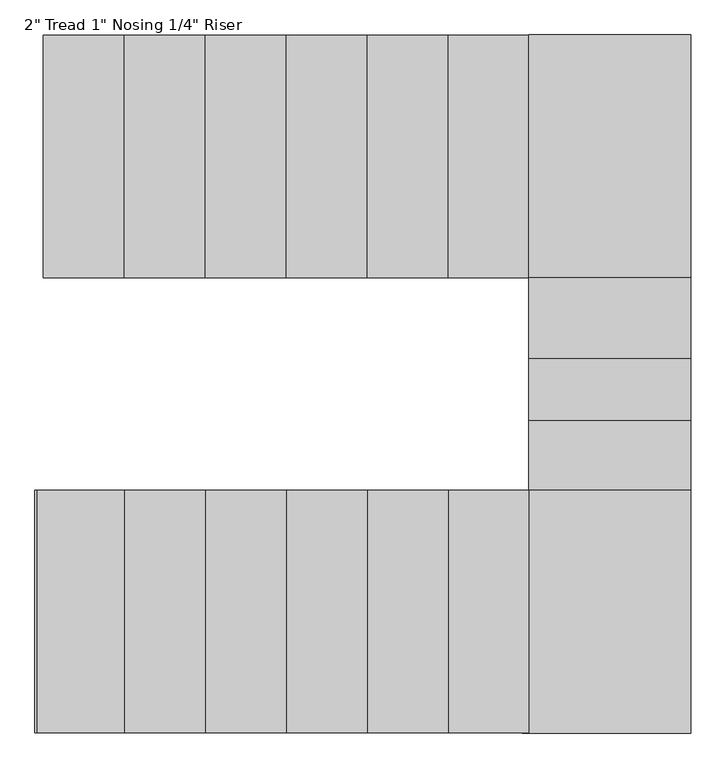
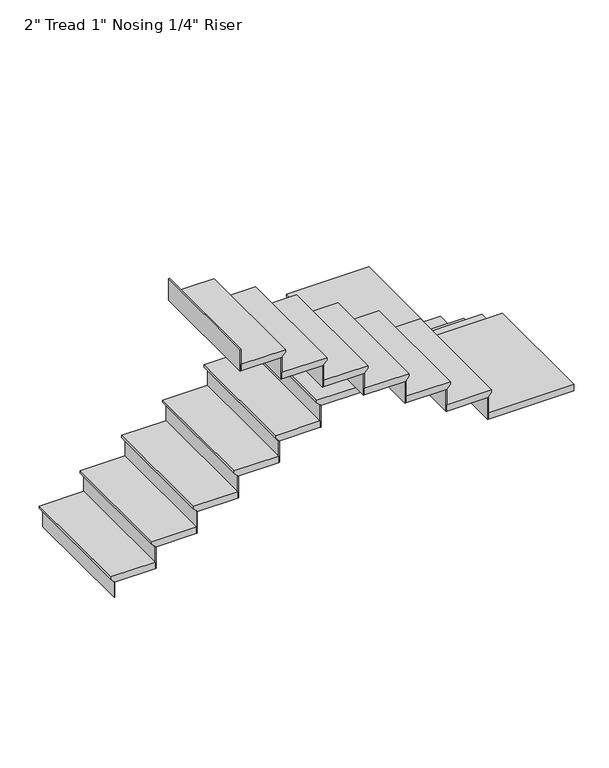
"""IFC4 building model written with IfcOpenShell, lengths in millimetres: stair flight geometry."""

from ifc_helpers import new_model, si_unit, origin, place, context, project, spatial, faceted_brep, source, transform, mapped, element, save


def stair_flight_9a0573e1(model_context):
    return source(origin(), model_context, "Body", "Brep", [
        faceted_brep([(6477.0, 10054.8323212, 9294.2833333), (6477.0, 10054.8323212, 9313.3333333), (6477.0, 10969.2323212, 9313.3333333), (6477.0, 10969.2323212, 9294.2833333), (6502.4, 10054.8323212, 9268.8833333), (6502.4, 10969.2323212, 9268.8833333), (6807.2, 10054.8323212, 9313.3333333), (6807.2, 10969.2323212, 9313.3333333), (6502.4, 10969.2323212, 9262.5333333), (6807.2, 10969.2323212, 9262.5333333), (6807.2, 10054.8323212, 9262.5333333), (6502.4, 10054.8323212, 9262.5333333)], [[[0, 1, 2, 3]], [[4, 0, 3, 5]], [[2, 1, 6, 7]], [[8, 9, 10, 11]], [[2, 7, 9, 8, 5, 3]], [[8, 11, 4, 5]], [[6, 1, 0, 4, 11, 10]], [[7, 6, 10, 9]]]),
        faceted_brep([(6502.4, 10054.8323212, 9262.5333333), (6502.4, 10054.8323212, 9144.0), (6508.75, 10054.8323212, 9144.0), (6508.75, 10054.8323212, 9262.5333333), (6502.4, 10969.2323212, 9262.5333333), (6508.75, 10969.2323212, 9262.5333333), (6508.75, 10969.2323212, 9144.0), (6502.4, 10969.2323212, 9144.0)], [[[0, 1, 2, 3]], [[4, 5, 6, 7]], [[1, 0, 4, 7]], [[2, 1, 7, 6]], [[3, 2, 6, 5]], [[0, 3, 5, 4]]]),
        faceted_brep([(6807.2, 10054.8323212, 9431.8666667), (6807.2, 10054.8323212, 9262.5333333), (6813.55, 10054.8323212, 9262.5333333), (6813.55, 10054.8323212, 9431.8666667), (6807.2, 10969.2323212, 9431.8666667), (6813.55, 10969.2323212, 9431.8666667), (6813.55, 10969.2323212, 9262.5333333), (6807.2, 10969.2323212, 9262.5333333)], [[[0, 1, 2, 3]], [[4, 5, 6, 7]], [[1, 0, 4, 7]], [[2, 1, 7, 6]], [[3, 2, 6, 5]], [[0, 3, 5, 4]]]),
        faceted_brep([(6781.8, 10969.2323212, 9482.6666667), (6781.8, 10054.8323212, 9482.6666667), (7112.0, 10054.8323212, 9482.6666667), (7112.0, 10969.2323212, 9482.6666667), (6807.2, 10969.2323212, 9431.8666667), (7112.0, 10969.2323212, 9431.8666667), (7112.0, 10054.8323212, 9431.8666667), (6807.2, 10054.8323212, 9431.8666667), (6807.2, 10969.2323212, 9438.2166667), (6781.8, 10969.2323212, 9463.6166667), (6807.2, 10054.8323212, 9438.2166667), (6781.8, 10054.8323212, 9463.6166667)], [[[0, 1, 2, 3]], [[4, 5, 6, 7]], [[0, 3, 5, 4, 8, 9]], [[4, 7, 10, 8]], [[2, 1, 11, 10, 7, 6]], [[3, 2, 6, 5]], [[11, 1, 0, 9]], [[10, 11, 9, 8]]]),
        faceted_brep([(7112.0, 10054.8323212, 9601.2), (7112.0, 10054.8323212, 9431.8666667), (7118.35, 10054.8323212, 9431.8666667), (7118.35, 10054.8323212, 9601.2), (7112.0, 10969.2323212, 9601.2), (7118.35, 10969.2323212, 9601.2), (7118.35, 10969.2323212, 9431.8666667), (7112.0, 10969.2323212, 9431.8666667)], [[[0, 1, 2, 3]], [[4, 5, 6, 7]], [[1, 0, 4, 7]], [[2, 1, 7, 6]], [[3, 2, 6, 5]], [[0, 3, 5, 4]]]),
        faceted_brep([(7086.6, 10969.2323212, 9652.0), (7086.6, 10054.8323212, 9652.0), (7416.8, 10054.8323212, 9652.0), (7416.8, 10969.2323212, 9652.0), (7112.0, 10969.2323212, 9601.2), (7416.8, 10969.2323212, 9601.2), (7416.8, 10054.8323212, 9601.2), (7112.0, 10054.8323212, 9601.2), (7112.0, 10969.2323212, 9607.55), (7086.6, 10969.2323212, 9632.95), (7112.0, 10054.8323212, 9607.55), (7086.6, 10054.8323212, 9632.95)], [[[0, 1, 2, 3]], [[4, 5, 6, 7]], [[0, 3, 5, 4, 8, 9]], [[4, 7, 10, 8]], [[2, 1, 11, 10, 7, 6]], [[3, 2, 6, 5]], [[11, 1, 0, 9]], [[10, 11, 9, 8]]]),
        faceted_brep([(7416.8, 10054.8323212, 9770.5333333), (7416.8, 10054.8323212, 9601.2), (7423.15, 10054.8323212, 9601.2), (7423.15, 10054.8323212, 9770.5333333), (7416.8, 10969.2323212, 9770.5333333), (7423.15, 10969.2323212, 9770.5333333), (7423.15, 10969.2323212, 9601.2), (7416.8, 10969.2323212, 9601.2)], [[[0, 1, 2, 3]], [[4, 5, 6, 7]], [[1, 0, 4, 7]], [[2, 1, 7, 6]], [[3, 2, 6, 5]], [[0, 3, 5, 4]]]),
        faceted_brep([(7391.4, 10969.2323212, 9821.3333333), (7391.4, 10054.8323212, 9821.3333333), (7721.6, 10054.8323212, 9821.3333333), (7721.6, 10969.2323212, 9821.3333333), (7416.8, 10969.2323212, 9770.5333333), (7721.6, 10969.2323212, 9770.5333333), (7721.6, 10054.8323212, 9770.5333333), (7416.8, 10054.8323212, 9770.5333333), (7416.8, 10969.2323212, 9776.8833333), (7391.4, 10969.2323212, 9802.2833333), (7416.8, 10054.8323212, 9776.8833333), (7391.4, 10054.8323212, 9802.2833333)], [[[0, 1, 2, 3]], [[4, 5, 6, 7]], [[0, 3, 5, 4, 8, 9]], [[4, 7, 10, 8]], [[2, 1, 11, 10, 7, 6]], [[3, 2, 6, 5]], [[11, 1, 0, 9]], [[10, 11, 9, 8]]]),
        faceted_brep([(7721.6, 10054.8323212, 9939.8666667), (7721.6, 10054.8323212, 9770.5333333), (7727.95, 10054.8323212, 9770.5333333), (7727.95, 10054.8323212, 9939.8666667), (7721.6, 10969.2323212, 9939.8666667), (7727.95, 10969.2323212, 9939.8666667), (7727.95, 10969.2323212, 9770.5333333), (7721.6, 10969.2323212, 9770.5333333)], [[[0, 1, 2, 3]], [[4, 5, 6, 7]], [[1, 0, 4, 7]], [[2, 1, 7, 6]], [[3, 2, 6, 5]], [[0, 3, 5, 4]]]),
        faceted_brep([(7696.2, 10969.2323212, 9990.6666667), (7696.2, 10054.8323212, 9990.6666667), (8026.4, 10054.8323212, 9990.6666667), (8026.4, 10969.2323212, 9990.6666667), (7721.6, 10969.2323212, 9939.8666667), (8026.4, 10969.2323212, 9939.8666667), (8026.4, 10054.8323212, 9939.8666667), (7721.6, 10054.8323212, 9939.8666667), (7721.6, 10969.2323212, 9946.2166667), (7696.2, 10969.2323212, 9971.6166667), (7721.6, 10054.8323212, 9946.2166667), (7696.2, 10054.8323212, 9971.6166667)], [[[0, 1, 2, 3]], [[4, 5, 6, 7]], [[0, 3, 5, 4, 8, 9]], [[4, 7, 10, 8]], [[2, 1, 11, 10, 7, 6]], [[3, 2, 6, 5]], [[11, 1, 0, 9]], [[10, 11, 9, 8]]]),
        faceted_brep([(8026.4, 10054.8323212, 10109.2), (8026.4, 10054.8323212, 9939.8666667), (8032.75, 10054.8323212, 9939.8666667), (8032.75, 10054.8323212, 10109.2), (8026.4, 10969.2323212, 10109.2), (8032.75, 10969.2323212, 10109.2), (8032.75, 10969.2323212, 9939.8666667), (8026.4, 10969.2323212, 9939.8666667)], [[[0, 1, 2, 3]], [[4, 5, 6, 7]], [[1, 0, 4, 7]], [[2, 1, 7, 6]], [[3, 2, 6, 5]], [[0, 3, 5, 4]]]),
        faceted_brep([(8001.0, 10969.2323212, 10160.0), (8001.0, 10054.8323212, 10160.0), (8331.2, 10054.8323212, 10160.0), (8331.2, 10969.2323212, 10160.0), (8026.4, 10969.2323212, 10109.2), (8331.2, 10969.2323212, 10109.2), (8331.2, 10054.8323212, 10109.2), (8026.4, 10054.8323212, 10109.2), (8026.4, 10969.2323212, 10115.55), (8001.0, 10969.2323212, 10140.95), (8026.4, 10054.8323212, 10115.55), (8001.0, 10054.8323212, 10140.95)], [[[0, 1, 2, 3]], [[4, 5, 6, 7]], [[0, 3, 5, 4, 8, 9]], [[4, 7, 10, 8]], [[2, 1, 11, 10, 7, 6]], [[3, 2, 6, 5]], [[11, 1, 0, 9]], [[10, 11, 9, 8]]]),
        faceted_brep([(8331.2, 10054.8323212, 10278.5333333), (8331.2, 10054.8323212, 10109.2), (8337.55, 10054.8323212, 10109.2), (8337.55, 10054.8323212, 10278.5333333), (8331.2, 10969.2323212, 10278.5333333), (8337.55, 10969.2323212, 10278.5333333), (8337.55, 10969.2323212, 10109.2), (8331.2, 10969.2323212, 10109.2)], [[[0, 1, 2, 3]], [[4, 5, 6, 7]], [[1, 0, 4, 7]], [[2, 1, 7, 6]], [[3, 2, 6, 5]], [[0, 3, 5, 4]]]),
        faceted_brep([(8915.4, 10029.4323212, 10329.3333333), (8915.4, 10969.2323212, 10329.3333333), (8305.8, 10969.2323212, 10329.3333333), (8305.8, 10029.4323212, 10329.3333333), (8915.4, 10969.2323212, 10278.5333333), (8915.4, 10029.4323212, 10278.5333333), (8305.8, 10029.4323212, 10278.5333333), (8305.8, 10054.8323212, 10278.5333333), (8331.2, 10054.8323212, 10278.5333333), (8331.2, 10969.2323212, 10278.5333333), (8331.2, 10969.2323212, 10284.8833333), (8305.8, 10969.2323212, 10310.2833333), (8331.2, 10054.8323212, 10284.8833333), (8305.8, 10054.8323212, 10310.2833333)], [[[0, 1, 2, 3]], [[4, 5, 6, 7, 8, 9]], [[1, 0, 5, 4]], [[2, 1, 4, 9, 10, 11]], [[9, 8, 12, 10]], [[8, 7, 13, 12]], [[3, 2, 11, 13, 7, 6]], [[0, 3, 6, 5]], [[11, 10, 12, 13]]]),
        faceted_brep([(8305.8, 10029.4323212, 10447.8666667), (8305.8, 10029.4323212, 10278.5333333), (8305.8, 10023.0823212, 10278.5333333), (8305.8, 10023.0823212, 10447.8666667), (8915.4, 10029.4323212, 10447.8666667), (8915.4, 10023.0823212, 10447.8666667), (8915.4, 10023.0823212, 10278.5333333), (8915.4, 10029.4323212, 10278.5333333)], [[[0, 1, 2, 3]], [[4, 5, 6, 7]], [[1, 0, 4, 7]], [[2, 1, 7, 6]], [[3, 2, 6, 5]], [[0, 3, 5, 4]]]),
        faceted_brep([(8915.4, 10054.8323212, 10498.6666667), (8305.8, 10054.8323212, 10498.6666667), (8305.8, 9724.6323212, 10498.6666667), (8915.4, 9724.6323212, 10498.6666667), (8915.4, 10029.4323212, 10447.8666667), (8915.4, 9724.6323212, 10447.8666667), (8305.8, 9724.6323212, 10447.8666667), (8305.8, 10029.4323212, 10447.8666667), (8915.4, 10029.4323212, 10454.2166667), (8915.4, 10054.8323212, 10479.6166667), (8305.8, 10029.4323212, 10454.2166667), (8305.8, 10054.8323212, 10479.6166667)], [[[0, 1, 2, 3]], [[4, 5, 6, 7]], [[0, 3, 5, 4, 8, 9]], [[4, 7, 10, 8]], [[2, 1, 11, 10, 7, 6]], [[3, 2, 6, 5]], [[11, 1, 0, 9]], [[10, 11, 9, 8]]]),
        faceted_brep([(8305.8, 9724.6323212, 10617.2), (8305.8, 9724.6323212, 10447.8666667), (8305.8, 9718.2823212, 10447.8666667), (8305.8, 9718.2823212, 10617.2), (8915.4, 9724.6323212, 10617.2), (8915.4, 9718.2823212, 10617.2), (8915.4, 9718.2823212, 10447.8666667), (8915.4, 9724.6323212, 10447.8666667)], [[[0, 1, 2, 3]], [[4, 5, 6, 7]], [[1, 0, 4, 7]], [[2, 1, 7, 6]], [[3, 2, 6, 5]], [[0, 3, 5, 4]]]),
        faceted_brep([(8915.4, 9750.0323212, 10668.0), (8305.8, 9750.0323212, 10668.0), (8305.8, 9491.8832929, 10668.0), (8915.4, 9491.8832929, 10668.0), (8915.4, 9724.6323212, 10617.2), (8915.4, 9491.8832929, 10617.2), (8305.8, 9491.8832929, 10617.2), (8305.8, 9724.6323212, 10617.2), (8915.4, 9724.6323212, 10623.55), (8915.4, 9750.0323212, 10648.95), (8305.8, 9724.6323212, 10623.55), (8305.8, 9750.0323212, 10648.95)], [[[0, 1, 2, 3]], [[4, 5, 6, 7]], [[0, 3, 5, 4, 8, 9]], [[4, 7, 10, 8]], [[2, 1, 11, 10, 7, 6]], [[3, 2, 6, 5]], [[11, 1, 0, 9]], [[10, 11, 9, 8]]]),
        faceted_brep([(8305.8, 9491.8832929, 10786.5333333), (8305.8, 9491.8832929, 10617.2), (8305.8, 9485.5332929, 10617.2), (8305.8, 9485.5332929, 10786.5333333), (8915.4, 9491.8832929, 10786.5333333), (8915.4, 9485.5332929, 10786.5333333), (8915.4, 9485.5332929, 10617.2), (8915.4, 9491.8832929, 10617.2)], [[[0, 1, 2, 3]], [[4, 5, 6, 7]], [[1, 0, 4, 7]], [[2, 1, 7, 6]], [[3, 2, 6, 5]], [[0, 3, 5, 4]]]),
        faceted_brep([(8915.4, 9517.2832929, 10837.3333333), (8305.8, 9517.2832929, 10837.3333333), (8305.8, 9229.3323212, 10837.3333333), (8915.4, 9229.3323212, 10837.3333333), (8915.4, 9491.8832929, 10786.5333333), (8915.4, 9229.3323212, 10786.5333333), (8305.8, 9229.3323212, 10786.5333333), (8305.8, 9491.8832929, 10786.5333333), (8915.4, 9491.8832929, 10792.8833333), (8915.4, 9517.2832929, 10818.2833333), (8305.8, 9491.8832929, 10792.8833333), (8305.8, 9517.2832929, 10818.2833333)], [[[0, 1, 2, 3]], [[4, 5, 6, 7]], [[0, 3, 5, 4, 8, 9]], [[4, 7, 10, 8]], [[2, 1, 11, 10, 7, 6]], [[3, 2, 6, 5]], [[11, 1, 0, 9]], [[10, 11, 9, 8]]]),
        faceted_brep([(8305.8, 9229.3323212, 10955.8666667), (8305.8, 9229.3323212, 10786.5333333), (8305.8, 9222.9823212, 10786.5333333), (8305.8, 9222.9823212, 10955.8666667), (8915.4, 9229.3323212, 10955.8666667), (8915.4, 9222.9823212, 10955.8666667), (8915.4, 9222.9823212, 10786.5333333), (8915.4, 9229.3323212, 10786.5333333)], [[[0, 1, 2, 3]], [[4, 5, 6, 7]], [[1, 0, 4, 7]], [[2, 1, 7, 6]], [[3, 2, 6, 5]], [[0, 3, 5, 4]]]),
        faceted_brep([(8280.4, 8340.3323212, 11006.6666667), (8915.4, 8340.3323212, 11006.6666667), (8915.4, 9254.7323212, 11006.6666667), (8280.4, 9254.7323212, 11006.6666667), (8915.4, 8340.3323212, 10955.8666667), (8280.4, 8340.3323212, 10955.8666667), (8280.4, 9254.7323212, 10955.8666667), (8305.8, 9254.7323212, 10955.8666667), (8305.8, 9229.3323212, 10955.8666667), (8915.4, 9229.3323212, 10955.8666667), (8915.4, 9229.3323212, 10962.2166667), (8915.4, 9254.7323212, 10987.6166667), (8305.8, 9229.3323212, 10962.2166667), (8305.8, 9254.7323212, 10987.6166667)], [[[0, 1, 2, 3]], [[4, 5, 6, 7, 8, 9]], [[1, 0, 5, 4]], [[2, 1, 4, 9, 10, 11]], [[9, 8, 12, 10]], [[8, 7, 13, 12]], [[3, 2, 11, 13, 7, 6]], [[0, 3, 6, 5]], [[11, 10, 12, 13]]]),
        faceted_brep([(8280.4, 9254.7323212, 11125.2), (8280.4, 9254.7323212, 10955.8666667), (8274.05, 9254.7323212, 10955.8666667), (8274.05, 9254.7323212, 11125.2), (8280.4, 8340.3323212, 11125.2), (8274.05, 8340.3323212, 11125.2), (8274.05, 8340.3323212, 10955.8666667), (8280.4, 8340.3323212, 10955.8666667)], [[[0, 1, 2, 3]], [[4, 5, 6, 7]], [[1, 0, 4, 7]], [[2, 1, 7, 6]], [[3, 2, 6, 5]], [[0, 3, 5, 4]]]),
        faceted_brep([(8305.8, 8340.3323212, 11176.0), (8305.8, 9254.7323212, 11176.0), (7975.6, 9254.7323212, 11176.0), (7975.6, 8340.3323212, 11176.0), (8280.4, 8340.3323212, 11125.2), (7975.6, 8340.3323212, 11125.2), (7975.6, 9254.7323212, 11125.2), (8280.4, 9254.7323212, 11125.2), (8280.4, 8340.3323212, 11131.55), (8305.8, 8340.3323212, 11156.95), (8280.4, 9254.7323212, 11131.55), (8305.8, 9254.7323212, 11156.95)], [[[0, 1, 2, 3]], [[4, 5, 6, 7]], [[0, 3, 5, 4, 8, 9]], [[4, 7, 10, 8]], [[2, 1, 11, 10, 7, 6]], [[3, 2, 6, 5]], [[11, 1, 0, 9]], [[10, 11, 9, 8]]]),
        faceted_brep([(7975.6, 9254.7323212, 11294.5333333), (7975.6, 9254.7323212, 11125.2), (7969.25, 9254.7323212, 11125.2), (7969.25, 9254.7323212, 11294.5333333), (7975.6, 8340.3323212, 11294.5333333), (7969.25, 8340.3323212, 11294.5333333), (7969.25, 8340.3323212, 11125.2), (7975.6, 8340.3323212, 11125.2)], [[[0, 1, 2, 3]], [[4, 5, 6, 7]], [[1, 0, 4, 7]], [[2, 1, 7, 6]], [[3, 2, 6, 5]], [[0, 3, 5, 4]]]),
        faceted_brep([(8001.0, 8340.3323212, 11345.3333333), (8001.0, 9254.7323212, 11345.3333333), (7670.8, 9254.7323212, 11345.3333333), (7670.8, 8340.3323212, 11345.3333333), (7975.6, 8340.3323212, 11294.5333333), (7670.8, 8340.3323212, 11294.5333333), (7670.8, 9254.7323212, 11294.5333333), (7975.6, 9254.7323212, 11294.5333333), (7975.6, 8340.3323212, 11300.8833333), (8001.0, 8340.3323212, 11326.2833333), (7975.6, 9254.7323212, 11300.8833333), (8001.0, 9254.7323212, 11326.2833333)], [[[0, 1, 2, 3]], [[4, 5, 6, 7]], [[0, 3, 5, 4, 8, 9]], [[4, 7, 10, 8]], [[2, 1, 11, 10, 7, 6]], [[3, 2, 6, 5]], [[11, 1, 0, 9]], [[10, 11, 9, 8]]]),
        faceted_brep([(7670.8, 9254.7323212, 11463.8666667), (7670.8, 9254.7323212, 11294.5333333), (7664.45, 9254.7323212, 11294.5333333), (7664.45, 9254.7323212, 11463.8666667), (7670.8, 8340.3323212, 11463.8666667), (7664.45, 8340.3323212, 11463.8666667), (7664.45, 8340.3323212, 11294.5333333), (7670.8, 8340.3323212, 11294.5333333)], [[[0, 1, 2, 3]], [[4, 5, 6, 7]], [[1, 0, 4, 7]], [[2, 1, 7, 6]], [[3, 2, 6, 5]], [[0, 3, 5, 4]]]),
        faceted_brep([(7696.2, 8340.3323212, 11514.6666667), (7696.2, 9254.7323212, 11514.6666667), (7366.0, 9254.7323212, 11514.6666667), (7366.0, 8340.3323212, 11514.6666667), (7670.8, 8340.3323212, 11463.8666667), (7366.0, 8340.3323212, 11463.8666667), (7366.0, 9254.7323212, 11463.8666667), (7670.8, 9254.7323212, 11463.8666667), (7670.8, 8340.3323212, 11470.2166667), (7696.2, 8340.3323212, 11495.6166667), (7670.8, 9254.7323212, 11470.2166667), (7696.2, 9254.7323212, 11495.6166667)], [[[0, 1, 2, 3]], [[4, 5, 6, 7]], [[0, 3, 5, 4, 8, 9]], [[4, 7, 10, 8]], [[2, 1, 11, 10, 7, 6]], [[3, 2, 6, 5]], [[11, 1, 0, 9]], [[10, 11, 9, 8]]]),
        faceted_brep([(7366.0, 9254.7323212, 11633.2), (7366.0, 9254.7323212, 11463.8666667), (7359.65, 9254.7323212, 11463.8666667), (7359.65, 9254.7323212, 11633.2), (7366.0, 8340.3323212, 11633.2), (7359.65, 8340.3323212, 11633.2), (7359.65, 8340.3323212, 11463.8666667), (7366.0, 8340.3323212, 11463.8666667)], [[[0, 1, 2, 3]], [[4, 5, 6, 7]], [[1, 0, 4, 7]], [[2, 1, 7, 6]], [[3, 2, 6, 5]], [[0, 3, 5, 4]]]),
        faceted_brep([(7391.4, 8340.3323212, 11684.0), (7391.4, 9254.7323212, 11684.0), (7061.2, 9254.7323212, 11684.0), (7061.2, 8340.3323212, 11684.0), (7366.0, 8340.3323212, 11633.2), (7061.2, 8340.3323212, 11633.2), (7061.2, 9254.7323212, 11633.2), (7366.0, 9254.7323212, 11633.2), (7366.0, 8340.3323212, 11639.55), (7391.4, 8340.3323212, 11664.95), (7366.0, 9254.7323212, 11639.55), (7391.4, 9254.7323212, 11664.95)], [[[0, 1, 2, 3]], [[4, 5, 6, 7]], [[0, 3, 5, 4, 8, 9]], [[4, 7, 10, 8]], [[2, 1, 11, 10, 7, 6]], [[3, 2, 6, 5]], [[11, 1, 0, 9]], [[10, 11, 9, 8]]]),
        faceted_brep([(7061.2, 9254.7323212, 11802.5333333), (7061.2, 9254.7323212, 11633.2), (7054.85, 9254.7323212, 11633.2), (7054.85, 9254.7323212, 11802.5333333), (7061.2, 8340.3323212, 11802.5333333), (7054.85, 8340.3323212, 11802.5333333), (7054.85, 8340.3323212, 11633.2), (7061.2, 8340.3323212, 11633.2)], [[[0, 1, 2, 3]], [[4, 5, 6, 7]], [[1, 0, 4, 7]], [[2, 1, 7, 6]], [[3, 2, 6, 5]], [[0, 3, 5, 4]]]),
        faceted_brep([(7086.6, 8340.3323212, 11853.3333333), (7086.6, 9254.7323212, 11853.3333333), (6756.4, 9254.7323212, 11853.3333333), (6756.4, 8340.3323212, 11853.3333333), (7061.2, 8340.3323212, 11802.5333333), (6756.4, 8340.3323212, 11802.5333333), (6756.4, 9254.7323212, 11802.5333333), (7061.2, 9254.7323212, 11802.5333333), (7061.2, 8340.3323212, 11808.8833333), (7086.6, 8340.3323212, 11834.2833333), (7061.2, 9254.7323212, 11808.8833333), (7086.6, 9254.7323212, 11834.2833333)], [[[0, 1, 2, 3]], [[4, 5, 6, 7]], [[0, 3, 5, 4, 8, 9]], [[4, 7, 10, 8]], [[2, 1, 11, 10, 7, 6]], [[3, 2, 6, 5]], [[11, 1, 0, 9]], [[10, 11, 9, 8]]]),
        faceted_brep([(6756.4, 9254.7323212, 11971.8666667), (6756.4, 9254.7323212, 11802.5333333), (6750.05, 9254.7323212, 11802.5333333), (6750.05, 9254.7323212, 11971.8666667), (6756.4, 8340.3323212, 11971.8666667), (6750.05, 8340.3323212, 11971.8666667), (6750.05, 8340.3323212, 11802.5333333), (6756.4, 8340.3323212, 11802.5333333)], [[[0, 1, 2, 3]], [[4, 5, 6, 7]], [[1, 0, 4, 7]], [[2, 1, 7, 6]], [[3, 2, 6, 5]], [[0, 3, 5, 4]]]),
        faceted_brep([(6451.6, 9254.7323212, 12141.2), (6451.6, 9254.7323212, 11971.8666667), (6445.25, 9254.7323212, 11971.8666667), (6445.25, 9254.7323212, 12141.2), (6451.6, 8340.3323212, 12141.2), (6445.25, 8340.3323212, 12141.2), (6445.25, 8340.3323212, 11971.8666667), (6451.6, 8340.3323212, 11971.8666667)], [[[0, 1, 2, 3]], [[4, 5, 6, 7]], [[1, 0, 4, 7]], [[2, 1, 7, 6]], [[3, 2, 6, 5]], [[0, 3, 5, 4]]]),
        faceted_brep([(6781.8, 8340.3323212, 12022.6666667), (6781.8, 9254.7323212, 12022.6666667), (6451.6, 9254.7323212, 12022.6666667), (6451.6, 8340.3323212, 12022.6666667), (6756.4, 8340.3323212, 11971.8666667), (6451.6, 8340.3323212, 11971.8666667), (6451.6, 9254.7323212, 11971.8666667), (6756.4, 9254.7323212, 11971.8666667), (6756.4, 8340.3323212, 11978.2166667), (6781.8, 8340.3323212, 12003.6166667), (6756.4, 9254.7323212, 11978.2166667), (6781.8, 9254.7323212, 12003.6166667)], [[[0, 1, 2, 3]], [[4, 5, 6, 7]], [[0, 3, 5, 4, 8, 9]], [[4, 7, 10, 8]], [[2, 1, 11, 10, 7, 6]], [[3, 2, 6, 5]], [[11, 1, 0, 9]], [[10, 11, 9, 8]]]),
    ])


if __name__ == "__main__":
    model = new_model("IFC4")
    model_context = context("Model", 3, world=origin())
    ifc_project = project(units=[si_unit("LENGTHUNIT", "METRE", prefix="MILLI")], contexts=[model_context])
    site = spatial("IfcSite", under=ifc_project)
    building = spatial("IfcBuilding", under=site)
    placement = place(None, origin())
    stair_flight_shape = stair_flight_9a0573e1(model_context)
    element("IfcStairFlight", 1, ObjectType="2\" Tread 1\" Nosing 1/4\" Riser", at=placement, inside=building, context=model_context, shape_type="MappedRepresentation", body=[
        mapped(stair_flight_shape, transform((0.0, 0.0, 0.0), x_axis=(1.0, 0.0, 0.0), y_axis=(0.0, 1.0, 0.0), z_axis=(0.0, 0.0, 1.0))),
    ])
    save(model, "model.ifc")
